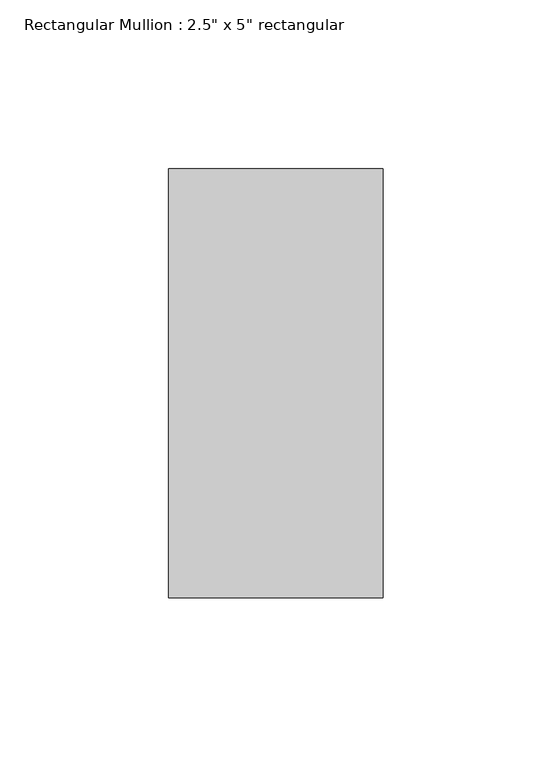
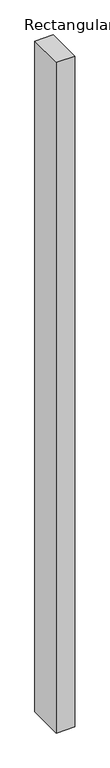
"""IFC4 building model written with IfcOpenShell, lengths in millimetres: member geometry."""

from ifc_helpers import new_model, si_unit, frame, origin, place, context, project, spatial, polyline, outline, extrude, source, transform, mapped, element, save


def member_f0fea5a5(model_context):
    return source(origin(), model_context, "Body", "SweptSolid", [
        extrude(outline(polyline([(31.75, 63.5), (31.75, -63.5), (-31.75, -63.5), (-31.75, 63.5), (31.75, 63.5)])), frame((0.0, 0.0, -2438.4), z_axis=(0.0, 0.0, 1.0), x_axis=(1.0, 0.0, 0.0)), (0.0, 0.0, 1.0), 2438.4),
    ])


if __name__ == "__main__":
    model = new_model("IFC4")
    model_context = context("Model", 3, world=origin())
    ifc_project = project(units=[si_unit("LENGTHUNIT", "METRE", prefix="MILLI")], contexts=[model_context])
    site = spatial("IfcSite", under=ifc_project)
    building = spatial("IfcBuilding", under=site)
    placement = place(None, origin())
    member_shape = member_f0fea5a5(model_context)
    element("IfcMember", 1, ObjectType="Rectangular Mullion : 2.5\" x 5\" rectangular", at=placement, inside=building, context=model_context, shape_type="MappedRepresentation", body=[
        mapped(member_shape, transform((0.0, 0.0, 0.0), x_axis=(1.0, 0.0, 0.0), y_axis=(0.0, 1.0, 0.0), z_axis=(0.0, 0.0, 1.0))),
    ])
    save(model, "model.ifc")

# Revit data of these elements
# Type "Rectangular Mullion : 2.5\" x 5\" rectangular"
#   built-in parameter 1007304 = 0.416667 (stored number, unit not read)
#   built-in parameter 1007301 = 0.104167 (stored number, unit not read)
#   built-in parameter 1007300 = 0.104167 (stored number, unit not read)
